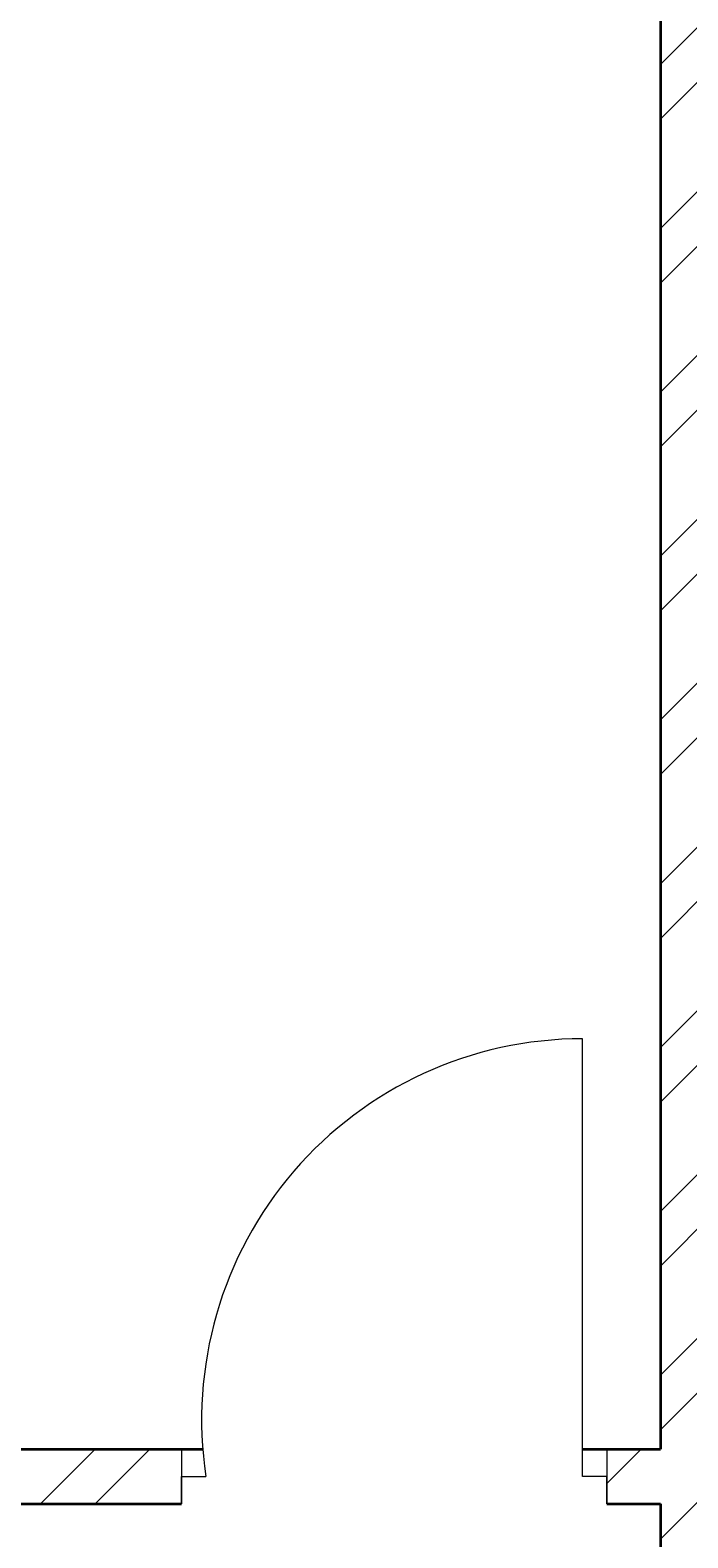
# Model space of a CAD drawing. Units: inches. Extents: x 1962 to 2771, y 1245 to 2660.
# Tile 108 of 114: x 2319 to 2374, y 2304 to 2428. Entities that reach past the tile are written whole.
import ezdxf

# ---------------------------------------------------------------- set-up
doc = ezdxf.new("R2010")
doc.units = ezdxf.units.IN
for name, color, linetype, lineweight in [('A-ANNO-DIMS', 2, 'Continuous', 18), ('A-DOOR', 3, 'Continuous', 18), ('A-WALL', 7, 'Continuous', 35), ('A-WALL-PATT', 252, 'Continuous', 13)]:
    doc.layers.add(name, color=color, linetype=linetype, lineweight=lineweight)
doc.styles.get("Standard").update_dxf_attribs({"font": 'arial.ttf'})
doc.dimstyles.get("Standard").update_dxf_attribs({"dimtxt": 0.18, "dimasz": 0.18, "dimexe": 0.18, "dimexo": 0.0625, "dimgap": 0.09, "dimtad": 0, "dimtih": 1, "dimtoh": 1, "dimdec": 4, "dimzin": 0, "dimdsep": 46, "dimtxsty": 'Standard', "dimcen": 0.09, "dimadec": 0, "dimazin": 0, "dimtfac": 1, "dimtdec": 4, "dimtofl": 0, "dimtmove": 0, "dimatfit": 3, "dimfxl": 1, "dimtolj": 1, "dimtzin": 0, "dimarcsym": 0})

# ---------------------------------------------------------------- blocks, each defined once
blk = doc.blocks.new('*D40')
at = {"layer": 'A-ANNO-DIMS', "color": 0, "lineweight": -2, "transparency": 16777216}
for p, q in [((2072.02, 2033.91), (2072.02, 2583.47)), ((2660.81, 2524.41), (2660.81, 2583.47)), ((2072.2, 2583.29), (2366.02, 2583.29)), ((2660.63, 2583.29), (2366.81, 2583.29))]:
    blk.add_line(p, q, dxfattribs=at)
at = {"layer": 'A-ANNO-DIMS', "color": 0, "transparency": 16777216}
for points in [[(2072.2, 2583.32), (2072.2, 2583.26), (2072.02, 2583.29)], [(2660.63, 2583.32), (2660.63, 2583.26), (2660.81, 2583.29)]]:
    blk.add_solid(points, dxfattribs=at)
at = {"layer": 'Defpoints', "color": 0, "transparency": 16777216}
for p in [(2660.81, 2583.29), (2660.81, 2524.34), (2072.02, 2033.84)]:
    blk.add_point(p, dxfattribs=at)
at = {"layer": 'A-ANNO-DIMS', "color": 0, "transparency": 16777216, "insert": (2366.41, 2583.29), "char_height": 0.18, "attachment_point": 5}
blk.add_mtext('\\A1;588.8', dxfattribs=at)

msp = doc.modelspace()

# ---------------------------------------------------------------- hatches: boundary and pattern name
at = {"layer": 'A-WALL-PATT'}
h = msp.add_hatch(dxfattribs=at)
h.set_pattern_fill('ANSI32', color=256)
h.paths.add_polyline_path([(2090.8074, 2467.3437), (2141.6481, 2467.3437), (2141.6481, 2469.5937), (2141.6481, 2471.8437), (2086.3074, 2471.8437), (2086.3074, 2422.5333), (2090.8074, 2422.5333)])
h.paths.add_polyline_path([(2282.7664, 2471.8437), (2204.8982, 2471.8437), (2204.8982, 2467.3437), (2234.8074, 2467.3437), (2234.8074, 2311.3437), (2228.7492, 2311.3437), (2228.7492, 2306.8437), (2234.8074, 2306.8437), (2331.9227, 2306.8437), (2331.9227, 2309.0937), (2331.9227, 2311.3437), (2239.3074, 2311.3437), (2239.3074, 2467.3437), (2282.7664, 2467.3437), (2282.7664, 2469.5937)])
h.paths.add_polyline_path([(2471.4531, 2519.8437), (2552.011, 2519.8437), (2564.3996, 2519.8437), (2564.3996, 2511.1389), (2568.8996, 2511.1389), (2568.8996, 2524.3437), (2466.9531, 2524.3437), (2466.9531, 2471.8437), (2450.0749, 2471.8437), (2446.4672, 2471.8437), (2446.4672, 2467.3437), (2450.0749, 2467.3437), (2475.9988, 2467.3437), (2475.9988, 2469.5937), (2475.9988, 2471.8437), (2471.4531, 2471.8437)])
h.paths.add_polyline_path([(2575.2231, 2469.5937), (2575.2231, 2471.8437), (2568.8996, 2471.8437), (2568.8996, 2487.1389), (2564.3996, 2487.1389), (2564.3996, 2471.8437), (2556.511, 2471.8437), (2499.2904, 2471.8437), (2499.2904, 2467.3437), (2507.8074, 2467.3437), (2507.8074, 2311.3437), (2414.863, 2311.3437), (2414.863, 2306.8437), (2512.3074, 2306.8437), (2517.0114, 2306.8437), (2517.0114, 2309.0937), (2517.0114, 2311.3437), (2512.3074, 2311.3437), (2512.3074, 2467.3437), (2575.2231, 2467.3437)])
h.paths.add_polyline_path([(2660.8074, 2471.8437), (2600.9602, 2471.8437), (2600.9602, 2467.3437), (2656.3074, 2467.3437), (2656.3074, 2432.5704), (2660.8074, 2432.5704)])
h.paths.add_polyline_path([(2660.8074, 2372.5704), (2656.3074, 2372.5704), (2656.3074, 2311.3437), (2600.276, 2311.3437), (2600.276, 2309.0937), (2600.276, 2306.8437), (2656.3074, 2306.8437), (2656.3074, 2296.2593), (2660.8074, 2296.2593)])
h.paths.add_polyline_path([(2572.3074, 2306.8437), (2577.1385, 2306.8437), (2577.1385, 2311.3437), (2551.082, 2311.3437), (2551.082, 2306.8437), (2567.8074, 2306.8437), (2567.8074, 2258.8437), (2540.0574, 2258.8437), (2540.0574, 2256.5937), (2540.0574, 2254.3437), (2567.8074, 2254.3437), (2656.3074, 2254.3437), (2656.3074, 2236.9085), (2660.8074, 2236.9085), (2660.8074, 2272.2593), (2656.3074, 2272.2593), (2656.3074, 2258.8437), (2572.3074, 2258.8437)])
h.paths.add_polyline_path([(2512.3074, 2254.3437), (2518.8716, 2254.3437), (2518.8716, 2256.5937), (2518.8716, 2258.8437), (2507.8074, 2258.8437), (2507.8074, 2177.8437), (2567.8074, 2177.8437), (2567.8074, 2172.9628), (2572.3074, 2172.9628), (2572.3074, 2177.8437), (2656.3074, 2177.8437), (2656.3074, 2166.4846), (2660.8074, 2166.4846), (2660.8074, 2200.9085), (2656.3074, 2200.9085), (2656.3074, 2182.3437), (2512.3074, 2182.3437)])
h.paths.add_polyline_path([(2656.3074, 2129.8437), (2572.3074, 2129.8437), (2572.3074, 2150.3044), (2570.0574, 2150.3044), (2567.8074, 2150.3044), (2567.8074, 2129.8437), (2507.8074, 2129.8437), (2507.8074, 2116.3027), (2510.0574, 2116.3027), (2512.3074, 2116.3027), (2512.3074, 2125.3437), (2567.8074, 2125.3437), (2572.3074, 2125.3437), (2656.3074, 2125.3437)])
h.paths.add_polyline_path([(2090.8074, 2362.5333), (2086.3074, 2362.5333), (2086.3074, 2298.6242), (2090.8074, 2298.6242), (2090.8074, 2306.8437), (2174.8074, 2306.8437), (2174.8074, 2286.4178), (2179.3074, 2286.4178), (2179.3074, 2306.8437), (2192.8641, 2306.8437), (2192.8641, 2309.0937), (2192.8641, 2311.3437), (2090.8074, 2311.3437)])
h.paths.add_polyline_path([(2209.156, 2258.8437), (2179.3074, 2258.8437), (2179.3074, 2263.2236), (2177.0574, 2263.2236), (2174.8074, 2263.2236), (2174.8074, 2258.8437), (2090.8074, 2258.8437), (2090.8074, 2274.6242), (2086.3074, 2274.6242), (2086.3074, 2238.2967), (2088.5574, 2238.2967), (2090.8074, 2238.2967), (2090.8074, 2254.3437), (2209.156, 2254.3437)])
h.paths.add_polyline_path([(2090.8074, 2177.8437), (2234.8074, 2177.8437), (2234.8074, 2173.1428), (2239.3074, 2173.1428), (2239.3074, 2258.8437), (2230.8442, 2258.8437), (2230.8442, 2256.5937), (2230.8442, 2254.3437), (2234.8074, 2254.3437), (2234.8074, 2182.3437), (2090.8074, 2182.3437), (2090.8074, 2202.2967), (2086.3074, 2202.2967), (2086.3074, 2140.0389), (2090.8074, 2140.0389)])
h.paths.add_polyline_path([(2090.8074, 2080.0389), (2086.3074, 2080.0389), (2086.3074, 2033.8437), (2090.8074, 2033.8437)], flags=17)
h.paths.add_polyline_path([(2244.9405, 2033.8437), (2239.3074, 2033.8437), (2239.3074, 2142.0665), (2237.2592, 2142.0665), (2234.8074, 2142.0665), (2234.8074, 2033.8437), (2090.8074, 2033.8437), (2076.5204, 2033.8437), (2072.0204, 2033.8437), (2072.0204, 2000.4493), (2076.5204, 2000.4493), (2076.5204, 2029.3437), (2090.8074, 2029.3437), (2244.9405, 2029.3437), (2244.9405, 2031.5937)])
h.paths.add_polyline_path([(2234.8074, 1933.3437), (2076.5204, 1933.3437), (2076.5204, 1952.4493), (2074.2704, 1952.4493), (2072.0204, 1952.4493), (2072.0204, 1933.3437), (2072.0204, 1928.8437), (2234.8074, 1928.8437)])
h.paths.add_polyline_path([(2090.8074, 1928.8437), (2086.3074, 1928.8437), (2086.3074, 1906.5013), (2090.8074, 1906.5013)])
h.paths.add_polyline_path([(2090.8074, 1846.5013), (2086.3074, 1846.5013), (2086.3074, 1769.9917), (2088.5574, 1769.9917), (2090.8074, 1769.9917), (2090.8074, 1780.3437), (2234.8074, 1780.3437), (2234.8074, 1708.3437), (2230.3764, 1708.3437), (2230.3764, 1703.8437), (2239.3074, 1703.8437), (2239.3074, 1792.6669), (2237.0574, 1792.6669), (2234.8074, 1792.6669), (2234.8074, 1784.8437), (2090.8074, 1784.8437)])
h.paths.add_polyline_path([(2239.3074, 1928.8437), (2244.9405, 1928.8437), (2244.9405, 1931.0937), (2244.9405, 1933.3437), (2234.8074, 1933.3437), (2234.8074, 1928.8437), (2234.8074, 1825.5949), (2239.3074, 1825.5949)])
h.paths.add_polyline_path([(2148.0425, 1649.0937), (2148.0425, 1651.3437), (2090.8074, 1651.3437), (2090.8074, 1646.8437), (2148.0425, 1646.8437)], flags=0)
h.paths.add_polyline_path([(2207.5601, 1708.3437), (2090.8074, 1708.3437), (2090.8074, 1703.8437), (2174.8074, 1703.8437), (2174.8074, 1651.3437), (2170.4457, 1651.3437), (2170.4457, 1646.8437), (2195.9924, 1646.8437), (2195.9924, 1649.0937), (2195.9924, 1651.3437), (2179.3074, 1651.3437), (2179.3074, 1703.8437), (2207.5601, 1703.8437), (2207.5601, 1706.0937)])
h.paths.add_polyline_path([(2090.8074, 1733.9917), (2086.3074, 1733.9917), (2086.3074, 1696.1032), (2088.5574, 1696.1032), (2090.8074, 1696.1032)])
h.paths.add_polyline_path([(2090.8074, 1672.1032), (2086.3074, 1672.1032), (2086.3074, 1600.3335), (2090.8074, 1600.3335)])
h.paths.add_polyline_path([(2090.8074, 1540.3335), (2086.3074, 1540.3335), (2086.3074, 1486.3437), (2139.6766, 1486.3437), (2139.6766, 1490.8437), (2090.8074, 1490.8437)])
h.paths.add_polyline_path([(2302.3876, 1490.8437), (2239.3074, 1490.8437), (2239.3074, 1646.8437), (2335.9994, 1646.8437), (2335.9994, 1651.3437), (2229.884, 1651.3437), (2229.884, 1646.8437), (2234.8074, 1646.8437), (2234.8074, 1490.8437), (2202.7103, 1490.8437), (2202.7103, 1488.5937), (2202.7103, 1486.3437), (2275.0699, 1486.3437), (2275.0699, 1475.772), (2279.5699, 1475.772), (2279.5699, 1486.3437), (2302.3876, 1486.3437)])
h.paths.add_polyline_path([(2279.5699, 1451.772), (2275.0699, 1451.772), (2275.0699, 1438.3437), (2174.8074, 1438.3437), (2174.8074, 1486.3437), (2179.7922, 1486.3437), (2179.7922, 1490.8437), (2163.3585, 1490.8437), (2163.3585, 1488.5937), (2163.3585, 1486.3437), (2170.3074, 1486.3437), (2170.3074, 1433.8437), (2279.5699, 1433.8437)])
h.paths.add_polyline_path([(2427.2363, 1490.8437), (2375.8074, 1490.8437), (2375.8074, 1646.8437), (2381.6401, 1646.8437), (2381.6401, 1651.3437), (2365.887, 1651.3437), (2365.887, 1649.0937), (2365.887, 1646.8437), (2371.3074, 1646.8437), (2371.3074, 1490.8437), (2327.5627, 1490.8437), (2327.5627, 1488.5937), (2327.5627, 1486.3437), (2371.3074, 1486.3437), (2371.3074, 1433.8437), (2375.8074, 1433.8437), (2375.8074, 1486.3437), (2427.2363, 1486.3437)])
h.paths.add_polyline_path([(2512.3074, 1646.8437), (2519.4351, 1646.8437), (2519.4351, 1649.0937), (2519.4351, 1651.3437), (2507.8074, 1651.3437), (2416.0063, 1651.3437), (2416.0063, 1649.0937), (2416.0063, 1646.8437), (2507.8074, 1646.8437), (2507.8074, 1490.8437), (2497.0532, 1490.8437), (2497.0532, 1488.5937), (2497.0532, 1486.3437), (2574.9344, 1486.3437), (2574.9344, 1476.0181), (2579.4344, 1476.0181), (2579.4344, 1486.3437), (2584.4872, 1486.3437), (2584.3074, 1490.8437), (2512.3074, 1490.8437)])
h.paths.add_polyline_path([(2470.5091, 1486.3437), (2473.9767, 1486.3437), (2473.9767, 1490.8437), (2449.6605, 1490.8437), (2449.6605, 1488.5937), (2449.6605, 1486.3437), (2466.0091, 1486.3437), (2466.0091, 1433.8437), (2470.5091, 1433.8437), (2579.4344, 1433.8437), (2579.4344, 1452.0181), (2574.9344, 1452.0181), (2574.9344, 1438.3437), (2554.5091, 1438.3437), (2470.5091, 1438.3437)])
h.paths.add_polyline_path([(2656.3074, 1490.8437), (2611.86, 1490.8437), (2611.86, 1486.3437), (2656.3074, 1486.3437)])
h.paths.add_polyline_path([(2660.8074, 1532.7007), (2658.5574, 1532.7007), (2656.3074, 1532.7007), (2656.3074, 1486.3437), (2660.8074, 1486.3437)])
h.paths.add_polyline_path([(2660.8074, 1664.9663), (2656.3074, 1664.9663), (2656.3074, 1651.3437), (2602.2313, 1651.3437), (2602.2313, 1646.8437), (2656.3074, 1646.8437), (2656.3074, 1592.7007), (2660.8074, 1592.7007)])
h.paths.add_polyline_path([(2660.8074, 1724.5221), (2656.3074, 1724.5221), (2656.3074, 1703.8437), (2542.4725, 1703.8437), (2542.4725, 1699.3437), (2567.8074, 1699.3437), (2567.8074, 1651.3437), (2552.7766, 1651.3437), (2552.7766, 1649.0937), (2552.7766, 1646.8437), (2577.2878, 1646.8437), (2577.2878, 1649.0937), (2577.2878, 1651.3437), (2572.3074, 1651.3437), (2572.3074, 1699.3437), (2656.3074, 1699.3437), (2656.3074, 1688.9663), (2660.8074, 1688.9663)])
h.paths.add_polyline_path([(2660.8074, 1880.6524), (2656.3074, 1880.6524), (2656.3074, 1832.8437), (2512.3074, 1832.8437), (2512.3074, 1837.8959), (2507.8074, 1837.8959), (2507.8074, 1828.3437), (2567.8074, 1828.3437), (2567.8074, 1804.3437), (2572.3074, 1804.3437), (2572.3074, 1828.3437), (2656.3074, 1828.3437), (2656.3074, 1818.6778), (2660.8074, 1818.6778)])
h.paths.add_polyline_path([(2660.8074, 1794.6778), (2656.3074, 1794.6778), (2656.3074, 1780.3437), (2572.3074, 1780.3437), (2572.3074, 1783.0303), (2570.0574, 1783.0303), (2567.8074, 1783.0303), (2567.8074, 1780.3437), (2507.8074, 1780.3437), (2507.8074, 1699.3437), (2517.8858, 1699.3437), (2517.8858, 1701.5937), (2517.8858, 1703.8437), (2512.3074, 1703.8437), (2512.3074, 1775.8437), (2656.3074, 1775.8437), (2656.3074, 1760.5221), (2660.8074, 1760.5221)])
h.paths.add_polyline_path([(2660.8074, 1981.3437), (2660.8074, 2020.2808), (2658.5574, 2020.2808), (2656.3074, 2020.2808), (2656.3074, 1981.3437), (2512.3074, 1981.3437), (2512.3074, 2086.6996), (2507.8074, 2086.6996), (2507.8074, 1981.3437), (2375.8074, 1981.3437), (2375.8074, 1986.8505), (2373.5574, 1986.8505), (2371.3074, 1986.8505), (2371.3074, 1973.2607), (2375.8074, 1973.2607), (2375.8074, 1976.8437), (2507.8074, 1976.8437), (2507.8074, 1865.4281), (2510.0574, 1865.4281), (2512.3074, 1865.4281), (2512.3074, 1976.8437), (2660.8074, 1976.8437)])
h.paths.add_polyline_path([(2375.8074, 1940.297), (2373.5574, 1940.297), (2371.3074, 1940.297), (2371.3074, 1933.3437), (2278.4434, 1933.3437), (2278.4434, 1928.8437), (2371.3074, 1928.8437), (2371.3074, 1651.3437), (2375.8074, 1651.3437)])
h.paths.add_polyline_path([(2660.8074, 1976.8437), (2656.3074, 1976.8437), (2656.3074, 1940.6524), (2660.8074, 1940.6524)], flags=17)
h.paths.add_polyline_path([(2660.8074, 2142.4846), (2656.3074, 2142.4846), (2656.3074, 2080.2808), (2660.8074, 2080.2808)])
h.paths.add_polyline_path([(2381.4189, 2311.3437), (2375.8074, 2311.3437), (2375.8074, 2467.3437), (2424.7242, 2467.3437), (2424.7242, 2469.5937), (2424.7242, 2471.8437), (2375.8074, 2471.8437), (2375.8074, 2524.3437), (2371.3074, 2524.3437), (2371.3074, 2471.8437), (2307.2097, 2471.8437), (2307.2097, 2467.3437), (2371.3074, 2467.3437), (2371.3074, 2311.3437), (2366.8901, 2311.3437), (2366.8901, 2306.8437), (2371.3074, 2306.8437), (2371.3074, 2033.8437), (2279.6589, 2033.8437), (2279.6589, 2029.3437), (2371.3074, 2029.3437), (2371.3074, 2014.2598), (2375.8074, 2014.2598), (2375.8074, 2306.8437), (2381.4189, 2306.8437)])
h.paths.add_polyline_path([(2263.3074, 2524.3437), (2170.3074, 2524.3437), (2170.3074, 2519.8437), (2170.3074, 2471.8437), (2165.0312, 2471.8437), (2165.0312, 2467.3437), (2179.6721, 2467.3437), (2179.6721, 2469.5161), (2179.6721, 2471.8437), (2174.8074, 2471.8437), (2174.8074, 2519.8437), (2258.8074, 2519.8437), (2258.8074, 2511.6436), (2263.3074, 2511.6436)])
h.paths.add_polyline_path([(2245.0232, 1361.4123), (2492.9468, 1361.4123), (2492.9468, 1398.505), (2245.0232, 1398.505)], flags=9)
h.paths.add_polyline_path([(2388.1434, 2086.6936), (2425.0704, 2086.6936), (2425.0704, 2105.3509), (2388.1434, 2105.3509)], flags=9)
h.paths.add_polyline_path([(2404.922, 2242.6744), (2445.7337, 2242.6744), (2445.7337, 2261.3318), (2404.922, 2261.3318)], flags=9)
h.paths.add_polyline_path([(2269.4107, 2156.7935), (2306.3378, 2156.7935), (2306.3378, 2175.4508), (2269.4107, 2175.4508)], flags=9)
h.paths.add_polyline_path([(2269.3277, 2233.4343), (2306.2547, 2233.4343), (2306.2547, 2252.0917), (2269.3277, 2252.0917)], flags=9)
h.paths.add_polyline_path([(2431.6052, 2320.6922), (2470.4456, 2320.6922), (2470.4456, 2339.3495), (2431.6052, 2339.3495)], flags=25)
h.paths.add_polyline_path([(2249.6902, 2315.7608), (2288.5306, 2315.7608), (2288.5306, 2334.4182), (2249.6902, 2334.4182)], flags=25)
h.paths.add_polyline_path([(2096.9301, 2314.3181), (2135.7704, 2314.3181), (2135.7704, 2332.9755), (2096.9301, 2332.9755)], flags=25)
h.paths.add_polyline_path([(2134.3475, 2285.7089), (2161.4655, 2285.7089), (2161.4655, 2304.3662), (2134.3475, 2304.3662)], flags=9)
h.paths.add_polyline_path([(2126.5155, 2209.4076), (2159.9227, 2209.4076), (2159.9227, 2228.065), (2126.5155, 2228.065)], flags=25)
h.paths.add_polyline_path([(2110.5753, 2141.5299), (2149.4157, 2141.5299), (2149.4157, 2160.1872), (2110.5753, 2160.1872)], flags=25)
h.paths.add_polyline_path([(2249.8618, 1968.3317), (2286.3966, 1968.3317), (2286.3966, 1986.989), (2249.8618, 1986.989)], flags=9)
h.paths.add_polyline_path([(2395.9507, 1777.0051), (2436.7624, 1777.0051), (2436.7624, 1795.6625), (2395.9507, 1795.6625)], flags=9)
h.paths.add_polyline_path([(2398.5259, 1888.5651), (2435.0062, 1888.5651), (2435.0062, 1907.2224), (2398.5259, 1907.2224)], flags=25)
h.paths.add_polyline_path([(2259.3506, 1728.3559), (2296.2776, 1728.3559), (2296.2776, 1747.0132), (2259.3506, 1747.0132)], flags=9)
h.paths.add_polyline_path([(2271.3698, 1845.268), (2308.2968, 1845.268), (2308.2968, 1863.9253), (2271.3698, 1863.9253)], flags=9)
h.paths.add_polyline_path([(2120.9355, 1786.3027), (2159.7759, 1786.3027), (2159.7759, 1804.9601), (2120.9355, 1804.9601)], flags=25)
h.paths.add_polyline_path([(2121.3164, 1732.1043), (2154.7236, 1732.1043), (2154.7236, 1750.7616), (2121.3164, 1750.7616)], flags=25)
h.paths.add_polyline_path([(2118.3706, 1678.8997), (2147.5282, 1678.8997), (2147.5282, 1697.557), (2118.3706, 1697.557)], flags=25)
h.paths.add_polyline_path([(2385.9227, 1493.557), (2424.763, 1493.557), (2424.763, 1512.2143), (2385.9227, 1512.2143)], flags=25)
h.paths.add_polyline_path([(2248.7058, 1500.0256), (2287.5462, 1500.0256), (2287.5462, 1518.6829), (2248.7058, 1518.6829)], flags=25)
h.paths.add_polyline_path([(2104.1669, 1617.3771), (2143.0073, 1617.3771), (2143.0073, 1636.0344), (2104.1669, 1636.0344)], flags=9)
h.paths.add_polyline_path([(2096.0714, 1447.8824), (2137.3845, 1447.8824), (2137.3845, 1458.1859), (2096.0714, 1458.1859)], flags=9)
h.paths.add_polyline_path([(2180.6114, 1440.325), (2209.7689, 1440.325), (2209.7689, 1458.9823), (2180.6114, 1458.9823)], flags=25)
h.paths.add_polyline_path([(2316.1698, 1447.9637), (2357.4829, 1447.9637), (2357.4829, 1458.2673), (2316.1698, 1458.2673)], flags=9)
h.paths.add_polyline_path([(2397.6187, 1447.9637), (2438.9318, 1447.9637), (2438.9318, 1458.2673), (2397.6187, 1458.2673)], flags=9)
h.paths.add_polyline_path([(2473.0778, 1439.5953), (2502.2354, 1439.5953), (2502.2354, 1458.2527), (2473.0778, 1458.2527)], flags=25)
h.paths.add_polyline_path([(2589.7027, 1447.8819), (2631.0158, 1447.8819), (2631.0158, 1458.1855), (2589.7027, 1458.1855)], flags=9)
h.paths.add_polyline_path([(2522.4009, 1497.5285), (2561.2413, 1497.5285), (2561.2413, 1516.1859), (2522.4009, 1516.1859)], flags=25)
h.paths.add_polyline_path([(2579.6565, 1671.3482), (2608.8141, 1671.3482), (2608.8141, 1690.0056), (2579.6565, 1690.0056)], flags=25)
h.paths.add_polyline_path([(2544.7038, 1725.5064), (2578.1111, 1725.5064), (2578.1111, 1744.1637), (2544.7038, 1744.1637)], flags=25)
h.paths.add_polyline_path([(2578.1191, 1807.472), (2607.2766, 1807.472), (2607.2766, 1826.1293), (2578.1191, 1826.1293)], flags=25)
h.paths.add_polyline_path([(2595.0614, 1835.1839), (2633.9018, 1835.1839), (2633.9018, 1853.8413), (2595.0614, 1853.8413)], flags=25)
h.paths.add_polyline_path([(2567.0097, 2097.7035), (2605.8501, 2097.7035), (2605.8501, 2116.3609), (2567.0097, 2116.3609)], flags=9)
h.paths.add_polyline_path([(2586.644, 2134.6454), (2615.8015, 2134.6454), (2615.8015, 2153.3027), (2586.644, 2153.3027)], flags=9)
h.paths.add_polyline_path([(2544.6185, 2212.6783), (2578.0258, 2212.6783), (2578.0258, 2231.3356), (2544.6185, 2231.3356)], flags=25)
h.paths.add_polyline_path([(2577.0273, 2256.9023), (2606.1849, 2256.9023), (2606.1849, 2275.5597), (2577.0273, 2275.5597)], flags=24)
h.paths.add_polyline_path([(2605.2683, 2315.2821), (2644.1087, 2315.2821), (2644.1087, 2333.9395), (2605.2683, 2333.9395)], flags=25)
h.paths.add_polyline_path([(2583.1244, 2496.1815), (2624.4375, 2496.1815), (2624.4375, 2506.4851), (2583.1244, 2506.4851)], flags=9)
h.paths.add_polyline_path([(2474.761, 2497.0823), (2503.9185, 2497.0823), (2503.9185, 2515.7397), (2474.761, 2515.7397)], flags=25)
h.paths.add_polyline_path([(2387.5787, 2494.2563), (2428.902, 2494.2563), (2428.902, 2504.5598), (2387.5787, 2504.5598)], flags=9)
h.paths.add_polyline_path([(2300.1657, 2500.1564), (2341.4788, 2500.1564), (2341.4788, 2510.46), (2300.1657, 2510.46)], flags=25)
h.paths.add_polyline_path([(2176.8589, 2497.5843), (2206.0165, 2497.5843), (2206.0165, 2516.2416), (2176.8589, 2516.2416)], flags=25)
h.paths.add_polyline_path([(2097.4668, 2494.9762), (2138.7799, 2494.9762), (2138.7799, 2505.2798), (2097.4668, 2505.2798)], flags=9)

# ---------------------------------------------------------------- linework, layer by layer
at = {"layer": 'A-DOOR'}
for p, q in [((2364.8901, 2309.0937), (2364.8901, 2345.0937)), ((2331.9227, 2311.3437), (2331.9227, 2306.8437)), ((2366.8901, 2311.3437), (2366.8901, 2306.8437)), ((2331.9227, 2306.8437), (2331.9227, 2309.0937)), ((2331.9227, 2309.0937), (2333.9227, 2309.0937)), ((2366.8901, 2309.0937), (2364.8901, 2309.0937)), ((2366.8901, 2306.8437), (2366.8901, 2309.0937))]:
    msp.add_line(p, q, dxfattribs=at)
msp.add_arc((2364.8901, 2313.7745), 31.3192, 90, 188.595327, dxfattribs=at)
at = {"layer": 'A-WALL'}
for p, q in [((2371.3074, 2467.3437), (2371.3074, 2311.3437)), ((2239.3074, 2311.3437), (2333.6654, 2311.3437)), ((2364.8901, 2311.3437), (2371.3074, 2311.3437)), ((2234.8074, 2306.8437), (2331.9227, 2306.8437)), ((2366.8901, 2306.8437), (2371.3074, 2306.8437)), ((2371.3074, 2306.8437), (2371.3074, 2033.8437))]:
    msp.add_line(p, q, dxfattribs=at)

# ---------------------------------------------------------------- dimensions: what is measured, and where the dimension line sits
at = {"layer": 'A-ANNO-DIMS'}
dim = msp.add_linear_dim(base=(2660.8074, 2583.2937), p1=(2072.0204, 2033.8437), p2=(2660.8074, 2524.3437), dimstyle='Standard', override={"dimdec": 1, "dimlfac": 1, "dimrnd": 0, "dimzin": 0, "dimdsep": 46, "dimlunit": 2}, dxfattribs=at)
dim.commit()
dim.dimension.update_dxf_attribs({"geometry": '*D40', "text_midpoint": (2366.4139, 2583.2937)})

doc.saveas('drawing.dxf')
